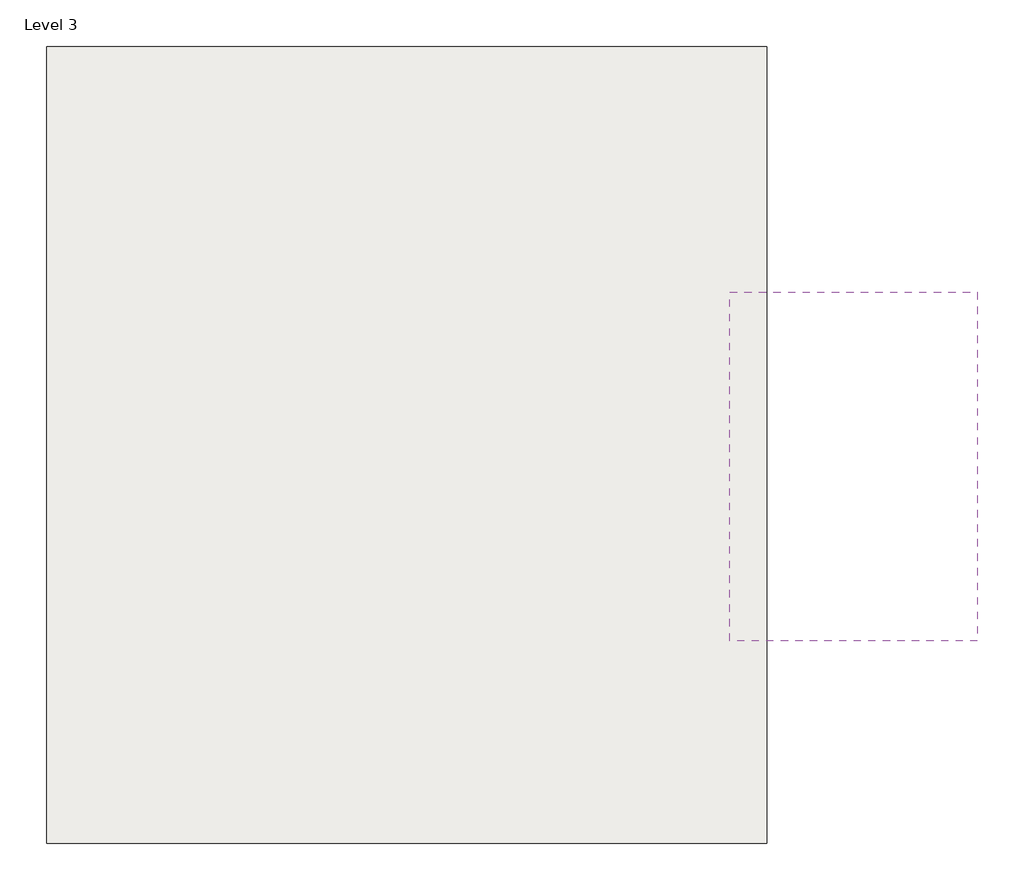
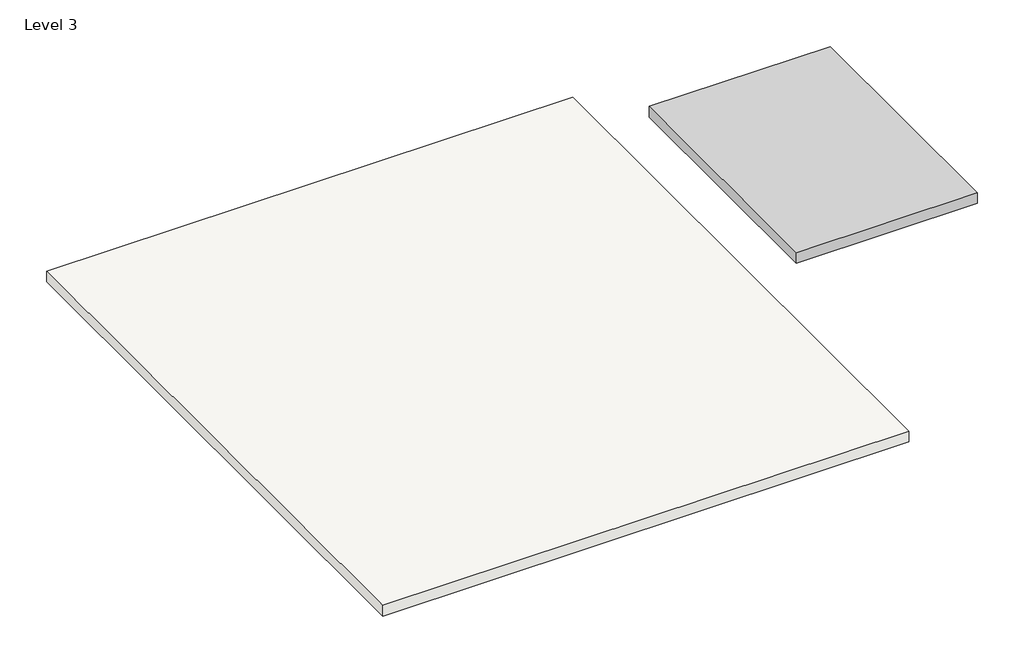
# One storey: 1 proxy, 1 roof.
"""IFC4 building model written with IfcOpenShell, lengths in millimetres."""

from ifc_helpers import new_model, si_unit, frame, origin, place, context, project, spatial, polyline, outline, extrude, transform, mapped, element, save
from components import generic_models_3_generic_models_3_5fb3f9a6

model = new_model("IFC4")

# Units and contexts
model_context = context("Model", 3, world=origin())
ifc_project = project(units=[si_unit("LENGTHUNIT", "METRE", prefix="MILLI")], contexts=[model_context])

# Site, building, storey
site = spatial("IfcSite", under=ifc_project)
building = spatial("IfcBuilding", under=site)
storey = spatial("IfcBuildingStorey", under=building, Name="Level 3", Elevation=6096.0)

# Proxy
placement = place(None, origin())
generic_models_3_generic_models_3_shape = generic_models_3_generic_models_3_5fb3f9a6(model_context)
element("IfcBuildingElementProxy", 1, Name="Generic Models 3 : Generic Models 3", ObjectType="Generic Models 3 : Generic Models 3", at=placement, inside=storey, context=model_context, shape_type="MappedRepresentation", body=[
    mapped(generic_models_3_generic_models_3_shape, transform((0.0, 0.0, 0.0), x_axis=(1.0, 0.0, 0.0), y_axis=(0.0, 1.0, 0.0), z_axis=(0.0, 0.0, 1.0))),
])

# Roof
element("IfcRoof", 2, ObjectType="Generic - 12\"", at=placement, inside=storey, context=model_context, shape_type="SweptSolid", body=[
    extrude(outline(polyline([(-20044.6120831, 3583.9054373), (-5871.4120831, 3583.9054373), (-5871.4120831, -12113.2945627), (-20044.6120831, -12113.2945627), (-20044.6120831, 3583.9054373)])), frame((0.0, 0.0, 6096.0), z_axis=(0.0, 0.0, 1.0), x_axis=(1.0, 0.0, 0.0)), (0.0, 0.0, 1.0), 304.8),
])

save(model, "model.ifc")

# Revit data of these elements
# Type "Generic - 12\""
#   Assembly Code = "B1020"
#   Layers, outside or top first: 1' - 0" no material (function 1)
# Element 1 (IfcBuildingElementProxy, "Generic Models 3 : Generic Models 3")
#   Phase Created = New Construction
# Element 2 (IfcRoof, "Generic - 12\"")
#   built-in parameter 1001705 = 21 (stored number, unit not read)
#   built-in parameter 1001710 = 33615
#   Phase Created = New Construction
#   Materials on its faces: "Default Roof"
# Materials
#   "Default Roof": colour RGB 88 101 114, transparency 0, Cost = 0
